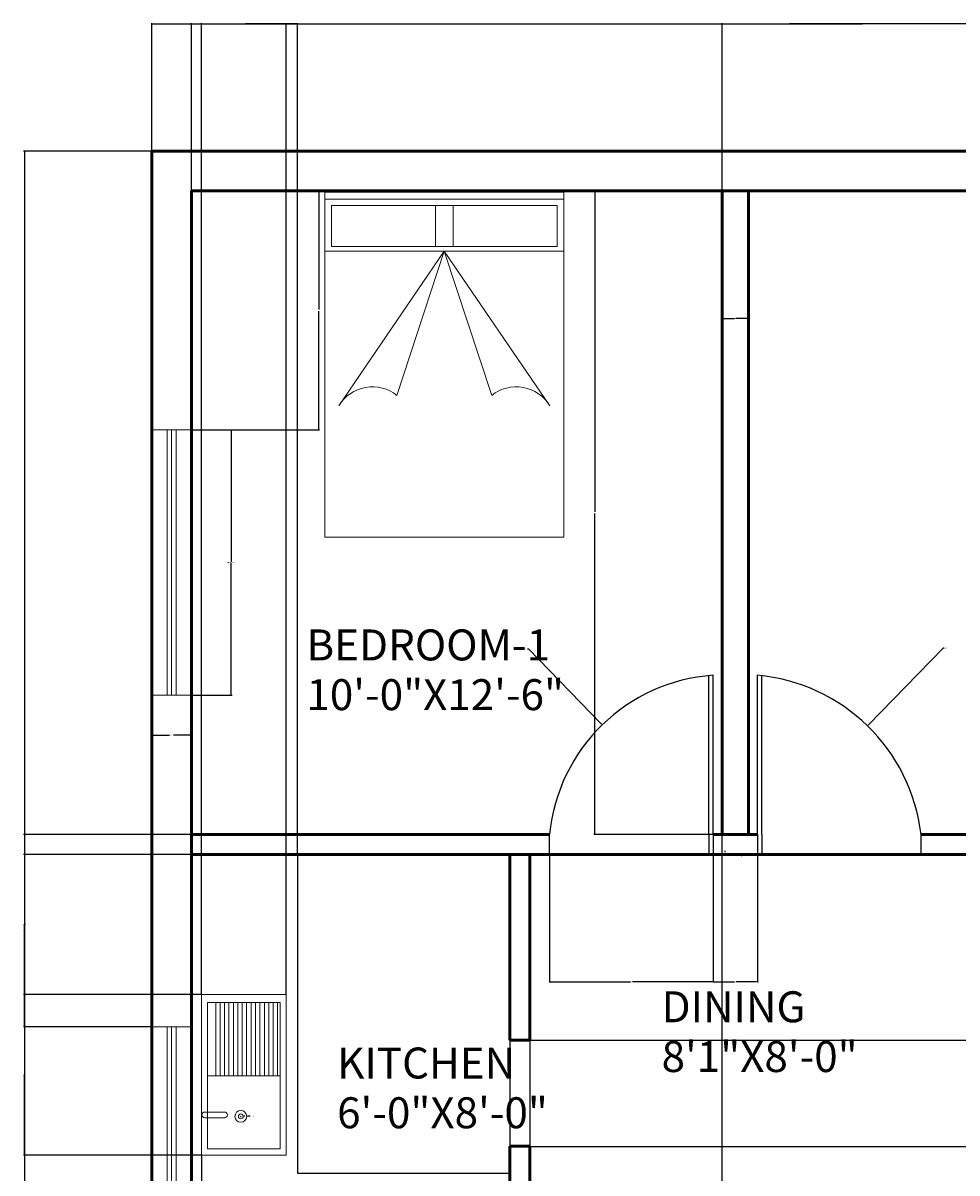
# Model space of a CAD drawing. Units: inches. Extents: x 2750 to 3097, y 1429 to 2028.
# Tile 3 of 4: x 2750 to 2962, y 1768 to 2028. Entities that reach past the tile are written whole.
import ezdxf

# ---------------------------------------------------------------- set-up
doc = ezdxf.new("R2010")
doc.units = ezdxf.units.IN
for name, color, linetype, lineweight in [('A-ANNO-DIMS', 2, 'Continuous', 18), ('A-AREA-IDEN', 7, 'Continuous', 25), ('A-DOOR', 3, 'Continuous', 25), ('A-FIXT-PATT', 252, 'Continuous', 13), ('A-FLOR-CASE', 8, 'Continuous', 25), ('A-FLOR-FIXT', 9, 'Continuous', 18), ('A-FURN', 8, 'Continuous', 18), ('A-GLAZ', 4, 'Continuous', 18), ('A-WALL', 7, 'Continuous', 50)]:
    doc.layers.add(name, color=color, linetype=linetype, lineweight=lineweight)
doc.styles.get("Standard").update_dxf_attribs({"font": 'arial.ttf'})
doc.dimstyles.get("Standard").update_dxf_attribs({"dimtxt": 0.18, "dimasz": 0.18, "dimexe": 0.18, "dimexo": 0.0625, "dimgap": 0.09, "dimtad": 0, "dimtih": 1, "dimtoh": 1, "dimdec": 4, "dimzin": 0, "dimdsep": 46, "dimtxsty": 'Standard', "dimcen": 0.09, "dimadec": 0, "dimazin": 0, "dimtfac": 1, "dimtdec": 4, "dimtofl": 0, "dimtmove": 0, "dimatfit": 3, "dimfxl": 1, "dimtolj": 1, "dimtzin": 0, "dimarcsym": 0})

# ---------------------------------------------------------------- blocks, each defined once
blk = doc.blocks.new('BED-DOUBLE-54X78')
for p, q in [((0, 78), (0, 0)), ((54, 78), (0, 78)), ((54, 0), (54, 78)), ((27, 13.39), (3.13, 48.31)), ((27, 13.39), (50.87, 48.31)), ((27, 13.39), (16.28, 45.98)), ((27, 13.39), (37.72, 45.98)), ((0, 13.39), (54, 13.39)), ((24.99, 3.04), (24.99, 12.35)), ((28.99, 3.04), (28.99, 12.35)), ((0, 1.59), (54, 1.59)), ((0, 0), (54, 0))]:
    blk.add_line(p, q)
blk.add_lwpolyline([(1.48, 3.04), (52.5, 3.04), (52.5, 12.35), (1.48, 12.35)], close=True)
for centre, start, end in [((10.73, 52.93), 211.2898, 308.6091), ((43.27, 52.93), 231.3909, 328.7102)]:
    blk.add_arc(centre, 8.89, start, end)
blk = doc.blocks.new('WIN-60IN')
for p, q in [((9, 60), (0, 60)), ((3.5, 60), (3.5, 0)), ((4.5, 60), (4.5, 0)), ((5.5, 60), (5.5, 0)), ((9, 0), (0, 0))]:
    blk.add_line(p, q)
blk = doc.blocks.new('WIN-36IN')
for p, q in [((9, 36), (0, 36)), ((3.5, 36), (3.5, 0)), ((4.5, 36), (4.5, 0)), ((5.5, 36), (5.5, 0)), ((9, 0), (0, 0))]:
    blk.add_line(p, q)
blk = doc.blocks.new('*D5')
at = {"layer": 'A-ANNO-DIMS', "color": 0, "lineweight": -2, "transparency": 16777216}
for p, q in [((2788.58, 1935.59), (2797.7, 1935.59)), ((2797.52, 1935.41), (2797.52, 1905.78)), ((2797.52, 1875.77), (2797.52, 1905.41)), ((2788.58, 1875.59), (2797.7, 1875.59))]:
    blk.add_line(p, q, dxfattribs=at)
at = {"layer": 'A-ANNO-DIMS', "color": 0, "transparency": 16777216}
for points in [[(2797.49, 1935.41), (2797.55, 1935.41), (2797.52, 1935.59)], [(2797.49, 1875.77), (2797.55, 1875.77), (2797.52, 1875.59)]]:
    blk.add_solid(points, dxfattribs=at)
at = {"layer": 'Defpoints', "color": 0, "transparency": 16777216}
for p in [(2788.52, 1935.59), (2797.52, 1935.59), (2788.52, 1875.59)]:
    blk.add_point(p, dxfattribs=at)
at = {"layer": 'A-ANNO-DIMS', "color": 0, "transparency": 16777216, "insert": (2797.52, 1905.59), "char_height": 0.18, "attachment_point": 5}
blk.add_mtext('\\A1;WINDOW 60 TYP.', dxfattribs=at)
blk = doc.blocks.new('*D6')
at = {"layer": 'A-ANNO-DIMS', "color": 0, "lineweight": -2, "transparency": 16777216}
for p, q in [((2779.52, 1875.53), (2779.52, 1866.41)), ((2788.52, 1875.53), (2788.52, 1866.41)), ((2779.7, 1866.59), (2783.56, 1866.59)), ((2788.34, 1866.59), (2784.48, 1866.59))]:
    blk.add_line(p, q, dxfattribs=at)
at = {"layer": 'A-ANNO-DIMS', "color": 0, "transparency": 16777216}
for points in [[(2779.7, 1866.62), (2779.7, 1866.56), (2779.52, 1866.59)], [(2788.34, 1866.62), (2788.34, 1866.56), (2788.52, 1866.59)]]:
    blk.add_solid(points, dxfattribs=at)
at = {"layer": 'Defpoints', "color": 0, "transparency": 16777216}
for p in [(2779.52, 1875.59), (2788.52, 1875.59), (2788.52, 1866.59)]:
    blk.add_point(p, dxfattribs=at)
at = {"layer": 'A-ANNO-DIMS', "color": 0, "transparency": 16777216, "insert": (2784.02, 1866.59), "char_height": 0.18, "attachment_point": 5}
blk.add_mtext('\\A1;9 TYP.', dxfattribs=at)
blk = doc.blocks.new('*D13')
at = {"layer": 'A-ANNO-DIMS', "color": 0, "lineweight": -2, "transparency": 16777216}
for p, q in [((2779.52, 1998.66), (2779.52, 2027.57)), ((2779.7, 2027.39), (2923.23, 2027.39)), ((3067.34, 2027.39), (2923.81, 2027.39)), ((3067.52, 1998.66), (3067.52, 2027.57))]:
    blk.add_line(p, q, dxfattribs=at)
at = {"layer": 'A-ANNO-DIMS', "color": 0, "transparency": 16777216}
for points in [[(2779.7, 2027.42), (2779.7, 2027.36), (2779.52, 2027.39)], [(3067.34, 2027.42), (3067.34, 2027.36), (3067.52, 2027.39)]]:
    blk.add_solid(points, dxfattribs=at)
at = {"layer": 'Defpoints', "color": 0, "transparency": 16777216}
for p in [(3067.52, 2027.39), (2779.52, 1998.59), (3067.52, 1998.59)]:
    blk.add_point(p, dxfattribs=at)
at = {"layer": 'A-ANNO-DIMS', "color": 0, "transparency": 16777216, "insert": (2923.52, 2027.39), "char_height": 0.18, "attachment_point": 5}
blk.add_mtext('\\A1;288', dxfattribs=at)
blk = doc.blocks.new('*D14')
at = {"layer": 'A-ANNO-DIMS', "color": 0, "lineweight": -2, "transparency": 16777216}
for p, q in [((2779.46, 1998.59), (2750.54, 1998.59)), ((2750.72, 1998.41), (2750.72, 1734.77)), ((2750.72, 1470.77), (2750.72, 1734.41)), ((2906.46, 1470.59), (2750.54, 1470.59))]:
    blk.add_line(p, q, dxfattribs=at)
at = {"layer": 'A-ANNO-DIMS', "color": 0, "transparency": 16777216}
for points in [[(2750.69, 1998.41), (2750.75, 1998.41), (2750.72, 1998.59)], [(2750.69, 1470.77), (2750.75, 1470.77), (2750.72, 1470.59)]]:
    blk.add_solid(points, dxfattribs=at)
at = {"layer": 'Defpoints', "color": 0, "transparency": 16777216}
for p in [(2750.72, 1998.59), (2779.52, 1998.59), (2906.52, 1470.59)]:
    blk.add_point(p, dxfattribs=at)
at = {"layer": 'A-ANNO-DIMS', "color": 0, "transparency": 16777216, "insert": (2750.72, 1734.59), "char_height": 0.18, "attachment_point": 5}
blk.add_mtext('\\A1;528', dxfattribs=at)
blk = doc.blocks.new('*D22')
at = {"layer": 'A-ANNO-DIMS', "color": 0, "lineweight": -2, "transparency": 16777216}
for p, q in [((2788.46, 1844.09), (2750.54, 1844.09)), ((2750.72, 1843.91), (2750.72, 1822.52)), ((2750.72, 1800.77), (2750.72, 1822.16)), ((2779.46, 1800.59), (2750.54, 1800.59))]:
    blk.add_line(p, q, dxfattribs=at)
at = {"layer": 'A-ANNO-DIMS', "color": 0, "transparency": 16777216}
for points in [[(2750.69, 1843.91), (2750.75, 1843.91), (2750.72, 1844.09)], [(2750.69, 1800.77), (2750.75, 1800.77), (2750.72, 1800.59)]]:
    blk.add_solid(points, dxfattribs=at)
at = {"layer": 'Defpoints', "color": 0, "transparency": 16777216}
for p in [(2788.52, 1844.09), (2750.72, 1800.59), (2779.52, 1800.59)]:
    blk.add_point(p, dxfattribs=at)
at = {"layer": 'A-ANNO-DIMS', "color": 0, "transparency": 16777216, "insert": (2750.72, 1822.34), "char_height": 0.18, "attachment_point": 5}
blk.add_mtext('\\A1;43.5', dxfattribs=at)
blk = doc.blocks.new('*D23')
at = {"layer": 'A-ANNO-DIMS', "color": 0, "lineweight": -2, "transparency": 16777216}
for p, q in [((2788.58, 1989.59), (2817.5, 1989.59)), ((2817.32, 1989.41), (2817.32, 1962.77)), ((2817.32, 1935.77), (2817.32, 1962.41)), ((2788.58, 1935.59), (2817.5, 1935.59))]:
    blk.add_line(p, q, dxfattribs=at)
at = {"layer": 'A-ANNO-DIMS', "color": 0, "transparency": 16777216}
for points in [[(2817.29, 1989.41), (2817.35, 1989.41), (2817.32, 1989.59)], [(2817.29, 1935.77), (2817.35, 1935.77), (2817.32, 1935.59)]]:
    blk.add_solid(points, dxfattribs=at)
at = {"layer": 'Defpoints', "color": 0, "transparency": 16777216}
for p in [(2788.52, 1989.59), (2788.52, 1935.59), (2817.32, 1935.59)]:
    blk.add_point(p, dxfattribs=at)
at = {"layer": 'A-ANNO-DIMS', "color": 0, "transparency": 16777216, "insert": (2817.32, 1962.59), "char_height": 0.18, "attachment_point": 5}
blk.add_mtext('\\A1;54', dxfattribs=at)
blk = doc.blocks.new('*D30')
at = {"layer": 'A-ANNO-DIMS', "color": 0, "lineweight": -2, "transparency": 16777216}
for p, q in [((2908.46, 1989.59), (2879.54, 1989.59)), ((2879.72, 1989.41), (2879.72, 1917.02)), ((2879.72, 1844.27), (2879.72, 1916.66)), ((2908.46, 1844.09), (2879.54, 1844.09))]:
    blk.add_line(p, q, dxfattribs=at)
at = {"layer": 'A-ANNO-DIMS', "color": 0, "transparency": 16777216}
for points in [[(2879.69, 1989.41), (2879.75, 1989.41), (2879.72, 1989.59)], [(2879.69, 1844.27), (2879.75, 1844.27), (2879.72, 1844.09)]]:
    blk.add_solid(points, dxfattribs=at)
at = {"layer": 'Defpoints', "color": 0, "transparency": 16777216}
for p in [(2879.72, 1989.59), (2908.52, 1989.59), (2908.52, 1844.09)]:
    blk.add_point(p, dxfattribs=at)
at = {"layer": 'A-ANNO-DIMS', "color": 0, "transparency": 16777216, "insert": (2879.72, 1916.84), "char_height": 0.18, "attachment_point": 5}
blk.add_mtext('\\A1;145.5', dxfattribs=at)
blk = doc.blocks.new('*D33')
at = {"layer": 'A-ANNO-DIMS', "color": 0, "lineweight": -2, "transparency": 16777216}
for p, q in [((2908.52, 1989.53), (2908.52, 1960.61)), ((2914.52, 1989.53), (2914.52, 1960.61)), ((2908.7, 1960.79), (2911.37, 1960.79)), ((2914.34, 1960.79), (2911.67, 1960.79))]:
    blk.add_line(p, q, dxfattribs=at)
at = {"layer": 'A-ANNO-DIMS', "color": 0, "transparency": 16777216}
for points in [[(2908.7, 1960.82), (2908.7, 1960.76), (2908.52, 1960.79)], [(2914.34, 1960.82), (2914.34, 1960.76), (2914.52, 1960.79)]]:
    blk.add_solid(points, dxfattribs=at)
at = {"layer": 'Defpoints', "color": 0, "transparency": 16777216}
for p in [(2908.52, 1989.59), (2914.52, 1989.59), (2908.52, 1960.79)]:
    blk.add_point(p, dxfattribs=at)
at = {"layer": 'A-ANNO-DIMS', "color": 0, "transparency": 16777216, "insert": (2911.52, 1960.79), "char_height": 0.18, "attachment_point": 5}
blk.add_mtext('\\A1;6', dxfattribs=at)
blk = doc.blocks.new('*D34')
at = {"layer": 'A-ANNO-DIMS', "color": 0, "lineweight": -2, "transparency": 16777216}
for p, q in [((2869.52, 1839.53), (2869.52, 1810.61)), ((2906.52, 1839.53), (2906.52, 1810.61)), ((2869.7, 1810.79), (2887.8, 1810.79)), ((2906.34, 1810.79), (2888.24, 1810.79))]:
    blk.add_line(p, q, dxfattribs=at)
at = {"layer": 'A-ANNO-DIMS', "color": 0, "transparency": 16777216}
for points in [[(2869.7, 1810.82), (2869.7, 1810.76), (2869.52, 1810.79)], [(2906.34, 1810.82), (2906.34, 1810.76), (2906.52, 1810.79)]]:
    blk.add_solid(points, dxfattribs=at)
at = {"layer": 'Defpoints', "color": 0, "transparency": 16777216}
for p in [(2869.52, 1839.59), (2906.52, 1839.59), (2869.52, 1810.79)]:
    blk.add_point(p, dxfattribs=at)
at = {"layer": 'A-ANNO-DIMS', "color": 0, "transparency": 16777216, "insert": (2888.02, 1810.79), "char_height": 0.18, "attachment_point": 5}
blk.add_mtext('\\A1;37', dxfattribs=at)
blk = doc.blocks.new('*D35')
at = {"layer": 'A-ANNO-DIMS', "color": 0, "lineweight": -2, "transparency": 16777216}
for p, q in [((2906.52, 1839.53), (2906.52, 1810.61)), ((2916.52, 1839.53), (2916.52, 1810.61)), ((2906.7, 1810.79), (2911.31, 1810.79)), ((2916.34, 1810.79), (2911.73, 1810.79))]:
    blk.add_line(p, q, dxfattribs=at)
at = {"layer": 'A-ANNO-DIMS', "color": 0, "transparency": 16777216}
for points in [[(2906.7, 1810.82), (2906.7, 1810.76), (2906.52, 1810.79)], [(2916.34, 1810.82), (2916.34, 1810.76), (2916.52, 1810.79)]]:
    blk.add_solid(points, dxfattribs=at)
at = {"layer": 'Defpoints', "color": 0, "transparency": 16777216}
for p in [(2906.52, 1839.59), (2916.52, 1839.59), (2906.52, 1810.79)]:
    blk.add_point(p, dxfattribs=at)
at = {"layer": 'A-ANNO-DIMS', "color": 0, "transparency": 16777216, "insert": (2911.52, 1810.79), "char_height": 0.18, "attachment_point": 5}
blk.add_mtext('\\A1;10', dxfattribs=at)
blk = doc.blocks.new('*D38')
at = {"layer": 'A-ANNO-DIMS', "color": 0, "lineweight": -2, "transparency": 16777216}
for p, q in [((2788.52, 1839.66), (2788.52, 2027.57)), ((2788.7, 2027.39), (2800.3, 2027.39)), ((2812.34, 2027.39), (2800.74, 2027.39)), ((2812.52, 1839.66), (2812.52, 2027.57))]:
    blk.add_line(p, q, dxfattribs=at)
at = {"layer": 'A-ANNO-DIMS', "color": 0, "transparency": 16777216}
for points in [[(2788.7, 2027.42), (2788.7, 2027.36), (2788.52, 2027.39)], [(2812.34, 2027.42), (2812.34, 2027.36), (2812.52, 2027.39)]]:
    blk.add_solid(points, dxfattribs=at)
at = {"layer": 'Defpoints', "color": 0, "transparency": 16777216}
for p in [(2812.52, 2027.39), (2788.52, 1839.59), (2812.52, 1839.59)]:
    blk.add_point(p, dxfattribs=at)
at = {"layer": 'A-ANNO-DIMS', "color": 0, "transparency": 16777216, "insert": (2800.52, 2027.39), "char_height": 0.18, "attachment_point": 5}
blk.add_mtext('\\A1;24', dxfattribs=at)
blk = doc.blocks.new('*D40')
at = {"layer": 'A-ANNO-DIMS', "color": 0, "lineweight": -2, "transparency": 16777216}
for p, q in [((2860.58, 1797.59), (3096.5, 1797.59)), ((3096.32, 1797.41), (3096.32, 1785.77)), ((3096.32, 1773.77), (3096.32, 1785.41)), ((2860.58, 1773.59), (3096.5, 1773.59))]:
    blk.add_line(p, q, dxfattribs=at)
at = {"layer": 'A-ANNO-DIMS', "color": 0, "transparency": 16777216}
for points in [[(3096.29, 1797.41), (3096.35, 1797.41), (3096.32, 1797.59)], [(3096.29, 1773.77), (3096.35, 1773.77), (3096.32, 1773.59)]]:
    blk.add_solid(points, dxfattribs=at)
at = {"layer": 'Defpoints', "color": 0, "transparency": 16777216}
for p in [(2860.52, 1797.59), (3096.32, 1797.59), (2860.52, 1773.59)]:
    blk.add_point(p, dxfattribs=at)
at = {"layer": 'A-ANNO-DIMS', "color": 0, "transparency": 16777216, "insert": (3096.32, 1785.59), "char_height": 0.18, "attachment_point": 5}
blk.add_mtext('\\A1;24', dxfattribs=at)
blk = doc.blocks.new('*D41')
at = {"layer": 'A-ANNO-DIMS', "color": 0, "lineweight": -2, "transparency": 16777216}
for p, q in [((2865.08, 1839.59), (3096.5, 1839.59)), ((3096.32, 1839.41), (3096.32, 1818.77)), ((3096.32, 1797.77), (3096.32, 1818.41)), ((2865.08, 1797.59), (3096.5, 1797.59))]:
    blk.add_line(p, q, dxfattribs=at)
at = {"layer": 'A-ANNO-DIMS', "color": 0, "transparency": 16777216}
for points in [[(3096.29, 1839.41), (3096.35, 1839.41), (3096.32, 1839.59)], [(3096.29, 1797.77), (3096.35, 1797.77), (3096.32, 1797.59)]]:
    blk.add_solid(points, dxfattribs=at)
at = {"layer": 'Defpoints', "color": 0, "transparency": 16777216}
for p in [(2865.02, 1839.59), (3096.32, 1839.59), (2865.02, 1797.59)]:
    blk.add_point(p, dxfattribs=at)
at = {"layer": 'A-ANNO-DIMS', "color": 0, "transparency": 16777216, "insert": (3096.32, 1818.59), "char_height": 0.18, "attachment_point": 5}
blk.add_mtext('\\A1;42', dxfattribs=at)
blk = doc.blocks.new('*D42')
at = {"layer": 'A-ANNO-DIMS', "color": 0, "lineweight": -2, "transparency": 16777216}
for p, q in [((2860.52, 1797.53), (2860.52, 1441.61)), ((2865.02, 1797.53), (2865.02, 1441.61)), ((2860.7, 1441.79), (2862.51, 1441.79)), ((2864.84, 1441.79), (2863.03, 1441.79))]:
    blk.add_line(p, q, dxfattribs=at)
at = {"layer": 'A-ANNO-DIMS', "color": 0, "transparency": 16777216}
for points in [[(2860.7, 1441.82), (2860.7, 1441.76), (2860.52, 1441.79)], [(2864.84, 1441.82), (2864.84, 1441.76), (2865.02, 1441.79)]]:
    blk.add_solid(points, dxfattribs=at)
at = {"layer": 'Defpoints', "color": 0, "transparency": 16777216}
for p in [(2860.52, 1797.59), (2865.02, 1797.59), (2865.02, 1441.79)]:
    blk.add_point(p, dxfattribs=at)
at = {"layer": 'A-ANNO-DIMS', "color": 0, "transparency": 16777216, "insert": (2862.77, 1441.79), "char_height": 0.18, "attachment_point": 5}
blk.add_mtext('\\A1;4.5', dxfattribs=at)
blk = doc.blocks.new('*D43')
at = {"layer": 'A-ANNO-DIMS', "color": 0, "lineweight": -2, "transparency": 16777216}
for p, q in [((2790.76, 1807.98), (2790.76, 2027.57)), ((2790.94, 2027.39), (2799.89, 2027.39)), ((2809.75, 2027.39), (2800.8, 2027.39)), ((2809.93, 1807.98), (2809.93, 2027.57))]:
    blk.add_line(p, q, dxfattribs=at)
at = {"layer": 'A-ANNO-DIMS', "color": 0, "transparency": 16777216}
for points in [[(2790.94, 2027.42), (2790.94, 2027.36), (2790.76, 2027.39)], [(2809.75, 2027.42), (2809.75, 2027.36), (2809.93, 2027.39)]]:
    blk.add_solid(points, dxfattribs=at)
at = {"layer": 'Defpoints', "color": 0, "transparency": 16777216}
for p in [(2809.93, 2027.39), (2790.76, 1807.91), (2809.93, 1807.91)]:
    blk.add_point(p, dxfattribs=at)
at = {"layer": 'A-ANNO-DIMS', "color": 0, "transparency": 16777216, "insert": (2800.34, 2027.39), "char_height": 0.18, "attachment_point": 5}
blk.add_mtext('\\A1;19.165', dxfattribs=at)
blk = doc.blocks.new('*D44')
at = {"layer": 'A-ANNO-DIMS', "color": 0, "lineweight": -2, "transparency": 16777216}
for p, q in [((2790.7, 1807.91), (2750.54, 1807.91)), ((2750.72, 1807.73), (2750.72, 1789.94)), ((2750.72, 1771.79), (2750.72, 1789.58)), ((2790.7, 1771.61), (2750.54, 1771.61))]:
    blk.add_line(p, q, dxfattribs=at)
at = {"layer": 'A-ANNO-DIMS', "color": 0, "transparency": 16777216}
for points in [[(2750.69, 1807.73), (2750.75, 1807.73), (2750.72, 1807.91)], [(2750.69, 1771.79), (2750.75, 1771.79), (2750.72, 1771.61)]]:
    blk.add_solid(points, dxfattribs=at)
at = {"layer": 'Defpoints', "color": 0, "transparency": 16777216}
for p in [(2750.72, 1807.91), (2790.76, 1807.91), (2790.76, 1771.61)]:
    blk.add_point(p, dxfattribs=at)
at = {"layer": 'A-ANNO-DIMS', "color": 0, "transparency": 16777216, "insert": (2750.72, 1789.76), "char_height": 0.18, "attachment_point": 5}
blk.add_mtext('\\A1;36.31', dxfattribs=at)
blk = doc.blocks.new('*D45')
at = {"layer": 'A-ANNO-DIMS', "color": 0, "lineweight": -2, "transparency": 16777216}
for p, q in [((2788.46, 1839.59), (2750.54, 1839.59)), ((2750.72, 1839.41), (2750.72, 1823.94)), ((2750.72, 1808.09), (2750.72, 1823.57)), ((2790.7, 1807.91), (2750.54, 1807.91))]:
    blk.add_line(p, q, dxfattribs=at)
at = {"layer": 'A-ANNO-DIMS', "color": 0, "transparency": 16777216}
for points in [[(2750.69, 1839.41), (2750.75, 1839.41), (2750.72, 1839.59)], [(2750.69, 1808.09), (2750.75, 1808.09), (2750.72, 1807.91)]]:
    blk.add_solid(points, dxfattribs=at)
at = {"layer": 'Defpoints', "color": 0, "transparency": 16777216}
for p in [(2788.52, 1839.59), (2750.72, 1807.91), (2790.76, 1807.91)]:
    blk.add_point(p, dxfattribs=at)
at = {"layer": 'A-ANNO-DIMS', "color": 0, "transparency": 16777216, "insert": (2750.72, 1823.75), "char_height": 0.18, "attachment_point": 5}
blk.add_mtext('\\A1;31.68', dxfattribs=at)
blk = doc.blocks.new('*D46')
at = {"layer": 'A-ANNO-DIMS', "color": 0, "lineweight": -2, "transparency": 16777216}
for p, q in [((2790.76, 1771.54), (2790.76, 1441.61)), ((2788.52, 1764.53), (2788.52, 1441.61)), ((2788.7, 1441.79), (2789.32, 1441.79)), ((2790.58, 1441.79), (2789.97, 1441.79))]:
    blk.add_line(p, q, dxfattribs=at)
at = {"layer": 'A-ANNO-DIMS', "color": 0, "transparency": 16777216}
for points in [[(2788.7, 1441.82), (2788.7, 1441.76), (2788.52, 1441.79)], [(2790.58, 1441.82), (2790.58, 1441.76), (2790.76, 1441.79)]]:
    blk.add_solid(points, dxfattribs=at)
at = {"layer": 'Defpoints', "color": 0, "transparency": 16777216}
for p in [(2790.76, 1771.61), (2788.52, 1764.59), (2790.76, 1441.79)]:
    blk.add_point(p, dxfattribs=at)
at = {"layer": 'A-ANNO-DIMS', "color": 0, "transparency": 16777216, "insert": (2789.64, 1441.79), "char_height": 0.18, "attachment_point": 5}
blk.add_mtext('\\A1;2.24', dxfattribs=at)
blk = doc.blocks.new('*D52')
at = {"layer": 'A-ANNO-DIMS', "color": 0, "lineweight": -2, "transparency": 16777216}
for p, q in [((2908.52, 1605.66), (2908.52, 2027.57)), ((2908.7, 2027.39), (2940.3, 2027.39)), ((2972.34, 2027.39), (2940.74, 2027.39)), ((2972.52, 1605.66), (2972.52, 2027.57))]:
    blk.add_line(p, q, dxfattribs=at)
at = {"layer": 'A-ANNO-DIMS', "color": 0, "transparency": 16777216}
for points in [[(2908.7, 2027.42), (2908.7, 2027.36), (2908.52, 2027.39)], [(2972.34, 2027.42), (2972.34, 2027.36), (2972.52, 2027.39)]]:
    blk.add_solid(points, dxfattribs=at)
at = {"layer": 'Defpoints', "color": 0, "transparency": 16777216}
for p in [(2972.52, 2027.39), (2908.52, 1605.59), (2972.52, 1605.59)]:
    blk.add_point(p, dxfattribs=at)
at = {"layer": 'A-ANNO-DIMS', "color": 0, "transparency": 16777216, "insert": (2940.52, 2027.39), "char_height": 0.18, "attachment_point": 5}
blk.add_mtext('\\A1;64', dxfattribs=at)
blk = doc.blocks.new('*D59')
at = {"layer": 'A-ANNO-DIMS', "color": 0, "lineweight": -2, "transparency": 16777216}
for p, q in [((2958.53, 1886.26), (2941.54, 1868.8)), ((2958.71, 1886.26), (2958.53, 1886.26)), ((2912.81, 1839.36), (2912.99, 1839.36)), ((2912.9, 1839.27), (2912.9, 1839.45))]:
    blk.add_line(p, q, dxfattribs=at)
at = {"layer": 'A-ANNO-DIMS', "color": 0, "transparency": 16777216}
blk.add_solid([(2941.52, 1868.82), (2941.57, 1868.78), (2941.42, 1868.67)], dxfattribs=at)
at = {"layer": 'Defpoints', "color": 0, "transparency": 16777216}
for p in [(2941.42, 1868.67), (2912.9, 1839.36)]:
    blk.add_point(p, dxfattribs=at)
at = {"layer": 'A-ANNO-DIMS', "color": 0, "transparency": 16777216, "insert": (2959.12, 1886.26), "char_height": 0.18, "attachment_point": 5}
blk.add_mtext('\\A1;R40.9', dxfattribs=at)
blk = doc.blocks.new('*D60')
at = {"layer": 'A-ANNO-DIMS', "color": 0, "lineweight": -2, "transparency": 16777216}
for p, q in [((2864.54, 1886.04), (2864.72, 1886.04)), ((2864.72, 1886.04), (2881.29, 1869.01)), ((2909.15, 1840.28), (2909.33, 1840.28)), ((2909.24, 1840.19), (2909.24, 1840.37))]:
    blk.add_line(p, q, dxfattribs=at)
at = {"layer": 'A-ANNO-DIMS', "color": 0, "transparency": 16777216}
blk.add_solid([(2881.31, 1869.03), (2881.27, 1868.99), (2881.41, 1868.88)], dxfattribs=at)
at = {"layer": 'Defpoints', "color": 0, "transparency": 16777216}
for p in [(2881.41, 1868.88), (2909.24, 1840.28)]:
    blk.add_point(p, dxfattribs=at)
at = {"layer": 'A-ANNO-DIMS', "color": 0, "transparency": 16777216, "insert": (2864.13, 1886.04), "char_height": 0.18, "attachment_point": 5}
blk.add_mtext('\\A1;R39.9', dxfattribs=at)
blk = doc.blocks.new('*D67')
at = {"layer": 'A-ANNO-DIMS', "color": 0, "lineweight": -2, "transparency": 16777216}
for p, q in [((2799.58, 1780.36), (2799.76, 1780.36)), ((2799.67, 1780.27), (2799.67, 1780.45)), ((2801.8, 1780.39), (2801.18, 1780.38))]:
    blk.add_line(p, q, dxfattribs=at)
at = {"layer": 'A-ANNO-DIMS', "color": 0, "transparency": 16777216}
blk.add_solid([(2801.18, 1780.41), (2801.18, 1780.35), (2801, 1780.38)], dxfattribs=at)
at = {"layer": 'Defpoints', "color": 0, "transparency": 16777216}
for p in [(2798.34, 1780.34), (2801, 1780.38)]:
    blk.add_point(p, dxfattribs=at)
at = {"layer": 'A-ANNO-DIMS', "color": 0, "transparency": 16777216, "insert": (2802.22, 1780.39), "char_height": 0.18, "attachment_point": 5}
blk.add_mtext('\\A1;∅2.66', dxfattribs=at)
blk = doc.blocks.new('*D68')
at = {"layer": 'A-ANNO-DIMS', "color": 0, "lineweight": -2, "transparency": 16777216}
for p, q in [((2799.58, 1780.36), (2799.76, 1780.36)), ((2799.67, 1780.27), (2799.67, 1780.45)), ((2800.58, 1780.39), (2800.4, 1780.39))]:
    blk.add_line(p, q, dxfattribs=at)
at = {"layer": 'A-ANNO-DIMS', "color": 0, "transparency": 16777216}
blk.add_solid([(2800.4, 1780.42), (2800.4, 1780.36), (2800.22, 1780.38)], dxfattribs=at)
at = {"layer": 'Defpoints', "color": 0, "transparency": 16777216}
for p in [(2799.12, 1780.34), (2800.22, 1780.38)]:
    blk.add_point(p, dxfattribs=at)
at = {"layer": 'A-ANNO-DIMS', "color": 0, "transparency": 16777216, "insert": (2801, 1780.39), "char_height": 0.18, "attachment_point": 5}
blk.add_mtext('\\A1;∅1.10', dxfattribs=at)

msp = doc.modelspace()

# ---------------------------------------------------------------- hatches: boundary and pattern name
at = {"layer": 'A-FIXT-PATT'}
h = msp.add_hatch(dxfattribs=at)
h.set_pattern_fill('ANSI31', color=256, scale=0.3149606, angle=45, style=0)
h.paths.add_polyline_path([(2793.1756, 1789.5616), (2808.1756, 1789.5616), (2808.1756, 1806.1191), (2793.1756, 1806.1191)])

# ---------------------------------------------------------------- linework, layer by layer
at = {"layer": 'A-DOOR'}
for p, q in [((2905.5201, 1844.0925), (2905.5201, 1880.0925)), ((2906.5201, 1844.0925), (2906.5201, 1880.0925)), ((2916.5201, 1844.0925), (2916.5201, 1880.0925)), ((2917.5201, 1844.0925), (2917.5201, 1880.0925)), ((2869.5201, 1839.5925), (2869.5201, 1844.0925)), ((2905.5201, 1844.0925), (2905.5201, 1839.5925)), ((2906.5201, 1844.0925), (2906.5201, 1839.5925)), ((2916.5201, 1844.0925), (2916.5201, 1839.5925)), ((2917.5201, 1844.0925), (2917.5201, 1839.5925)), ((2953.5201, 1839.5925), (2953.5201, 1844.0925)), ((2905.5201, 1839.5925), (2869.5201, 1839.5925)), ((2917.5201, 1839.5925), (2953.5201, 1839.5925))]:
    msp.add_line(p, q, dxfattribs=at)
for centre, radius, start, end in [((2909.2403, 1840.2829), 39.9025, 93.908995, 174.521356), ((2912.8987, 1839.3566), 40.8965, 6.649866, 84.919783)]:
    msp.add_arc(centre, radius, start, end, dxfattribs=at)
at = {"layer": 'A-FLOR-CASE'}
for p, q in [((2788.5201, 1839.5925), (2812.5201, 1839.5925)), ((2788.5201, 1839.5925), (2788.5201, 1815.5925)), ((2788.5201, 1839.5925), (2812.5201, 1839.5925)), ((2812.5201, 1839.5925), (2812.5201, 1767.5629)), ((2812.5201, 1767.5629), (2860.5201, 1767.5629))]:
    msp.add_line(p, q, dxfattribs=at)
at = {"layer": 'A-FLOR-FIXT'}
for p, q in [((2792.1775, 1789.5616), (2808.5798, 1789.5616)), ((2791.5203, 1781.3448), (2795.9949, 1781.3448)), ((2791.5203, 1781.3448), (2796.0603, 1781.3448)), ((2791.5203, 1780.0392), (2796.0603, 1780.0392)), ((2791.5203, 1780.0392), (2795.9949, 1780.0392))]:
    msp.add_line(p, q, dxfattribs=at)
for points in [[(2790.7618, 1807.9144), (2809.9266, 1807.9144), (2809.9266, 1771.6062), (2790.7618, 1771.6062)], [(2792.1775, 1806.1191), (2808.5798, 1806.1191), (2808.5798, 1773.0041), (2792.1775, 1773.0041)]]:
    msp.add_lwpolyline(points, close=True, dxfattribs=at)
for radius in [1.3318, 0.5481]:
    msp.add_circle((2799.6724, 1780.359), radius, dxfattribs=at)
for centre, start, end in [((2791.5203, 1780.692), 90, 270), ((2795.9949, 1780.692), 270, 90)]:
    msp.add_arc(centre, 0.6528, start, end, dxfattribs=at)
at = {"layer": 'A-GLAZ'}
for p, q in [((2784.0201, 1935.5925), (2788.5201, 1935.5925)), ((2784.0201, 1875.5925), (2788.5201, 1875.5925)), ((2784.0201, 1800.5925), (2788.5201, 1800.5925))]:
    msp.add_line(p, q, dxfattribs=at)
at = {"layer": 'A-WALL'}
for p, q in [((2779.5201, 1998.5925), (3067.5201, 1998.5925)), ((2779.5201, 1494.5925), (2779.5201, 1998.5925)), ((2788.5201, 1989.5925), (3058.5201, 1989.5925)), ((2788.5201, 1503.5925), (2788.5201, 1989.5925)), ((2908.5201, 1844.0925), (2908.5201, 1989.5925)), ((2914.5201, 1989.5925), (2914.5201, 1844.0925)), ((2788.5201, 1844.0925), (2869.5201, 1844.0925)), ((2908.5201, 1844.0925), (2906.5201, 1844.0925)), ((2906.5201, 1844.0925), (2916.5201, 1844.0925)), ((2914.5201, 1844.0925), (2916.5201, 1844.0925)), ((2953.5201, 1844.0925), (3058.5201, 1844.0925)), ((2788.5201, 1839.5925), (2965.0201, 1839.5925)), ((2860.5201, 1797.5925), (2860.5201, 1839.5925)), ((2865.0201, 1839.5925), (2865.0201, 1797.5925)), ((2865.0201, 1797.5925), (2865.0201, 1839.5925)), ((2865.0201, 1797.5925), (2860.5201, 1797.5925)), ((2860.5201, 1743.5925), (2860.5201, 1773.5925)), ((2860.5201, 1773.5925), (2865.0201, 1773.5925)), ((2865.0201, 1743.5925), (2865.0201, 1773.5925))]:
    msp.add_line(p, q, dxfattribs=at)

# ---------------------------------------------------------------- block references
at = {"layer": 'A-FURN', "rotation": 180}
msp.add_blockref('BED-DOUBLE-54X78', (2872.7026, 1989.3549), dxfattribs=at)
at = {"layer": 'A-GLAZ'}
for name, p in [('WIN-60IN', (2779.52, 1875.593)), ('WIN-36IN', (2779.52, 1764.593))]:
    msp.add_blockref(name, p, dxfattribs=at)

# ---------------------------------------------------------------- texts
at = {"layer": 'A-AREA-IDEN'}
for s, p in [('BEDROOM-1', (2814.5156, 1883.4577)), ('10\'-0"X12\'-6"', (2814.5156, 1872.2128)), ('DINING', (2894.848, 1801.639)), ('8\'1"X8\'-0"', (2894.848, 1790.3941)), ('KITCHEN', (2821.4628, 1788.9263)), ('6\'-0"X8\'-0"', (2821.4628, 1777.6814))]:
    msp.add_text(s, height=7, dxfattribs=at).set_placement(p)

# ---------------------------------------------------------------- dimensions: what is measured, and where the dimension line sits
at = {"layer": 'A-ANNO-DIMS'}
for base, p1, p2, override, picture, middle in [((3067.5201, 2027.3925), (2779.5201, 1998.5925), (3067.5201, 1998.5925), {"dimdec": 0, "dimlfac": 1, "dimrnd": 0, "dimzin": 0, "dimdsep": 46, "dimlunit": 2}, '*D13', (2923.5201, 2027.3925)), ((2812.5201, 2027.3925), (2788.5201, 1839.5925), (2812.5201, 1839.5925), {"dimdec": 0, "dimlfac": 1, "dimrnd": 0, "dimzin": 0, "dimdsep": 46, "dimlunit": 2}, '*D38', (2800.5201, 2027.3925)), ((2809.9266, 2027.3925), (2790.7618, 1807.9144), (2809.9266, 1807.9144), {"dimdec": 3, "dimlfac": 1, "dimrnd": 0, "dimzin": 0, "dimdsep": 46, "dimlunit": 2}, '*D43', (2800.3442, 2027.3925)), ((2972.5201, 2027.3925), (2908.5201, 1605.5925), (2972.5201, 1605.5925), {"dimdec": 0, "dimlfac": 1, "dimrnd": 0, "dimzin": 0, "dimdsep": 46, "dimlunit": 2}, '*D52', (2940.5201, 2027.3925)), ((2865.0201, 1441.7925), (2860.5201, 1797.5925), (2865.0201, 1797.5925), {"dimdec": 1, "dimlfac": 1, "dimrnd": 0, "dimzin": 0, "dimdsep": 46, "dimlunit": 2}, '*D42', (2862.7701, 1441.7925)), ((2790.7618, 1441.7925), (2788.5201, 1764.5925), (2790.7618, 1771.6062), {"dimdec": 2, "dimlfac": 1, "dimrnd": 0, "dimzin": 0, "dimdsep": 46, "dimlunit": 2}, '*D46', (2789.641, 1441.7925))]:
    dim = msp.add_linear_dim(base=base, p1=p1, p2=p2, dimstyle='Standard', override=override, dxfattribs=at)
    dim.commit()
    dim.dimension.update_dxf_attribs({"geometry": picture, "text_midpoint": middle})
for base, p1, p2, angle, override, picture, middle in [((2750.7201, 1998.5925), (2906.5201, 1470.5925), (2779.5201, 1998.5925), 90, {"dimdec": 0, "dimlfac": 1, "dimrnd": 0, "dimzin": 0, "dimdsep": 46, "dimlunit": 2}, '*D14', (2750.7201, 1734.5925)), ((2817.3201, 1935.5925), (2788.5201, 1989.5925), (2788.5201, 1935.5925), 270, {"dimdec": 0, "dimlfac": 1, "dimrnd": 0, "dimzin": 0, "dimdsep": 46, "dimlunit": 2}, '*D23', (2817.3201, 1962.5925)), ((2879.7201, 1989.5925), (2908.5201, 1844.0925), (2908.5201, 1989.5925), 90, {"dimdec": 1, "dimlfac": 1, "dimrnd": 0, "dimzin": 0, "dimdsep": 46, "dimlunit": 2}, '*D30', (2879.7201, 1916.8425)), ((2908.5201, 1960.7925), (2914.5201, 1989.5925), (2908.5201, 1989.5925), 180, {"dimdec": 0, "dimlfac": 1, "dimrnd": 0, "dimzin": 0, "dimdsep": 46, "dimlunit": 2}, '*D33', (2911.5201, 1960.7925)), ((2750.7201, 1800.5925), (2788.5201, 1844.0925), (2779.5201, 1800.5925), 90, {"dimdec": 1, "dimlfac": 1, "dimrnd": 0, "dimzin": 0, "dimdsep": 46, "dimlunit": 2}, '*D22', (2750.7201, 1822.3425)), ((2750.7201, 1807.9144), (2788.5201, 1839.5925), (2790.7618, 1807.9144), 90, {"dimdec": 2, "dimlfac": 1, "dimrnd": 0, "dimzin": 0, "dimdsep": 46, "dimlunit": 2}, '*D45', (2750.7201, 1823.7535)), ((3096.3201, 1839.5925), (2865.0201, 1797.5925), (2865.0201, 1839.5925), 90, {"dimdec": 0, "dimlfac": 1, "dimrnd": 0, "dimzin": 0, "dimdsep": 46, "dimlunit": 2}, '*D41', (3096.3201, 1818.5925)), ((2869.5201, 1810.7925), (2906.5201, 1839.5925), (2869.5201, 1839.5925), 180, {"dimdec": 0, "dimlfac": 1, "dimrnd": 0, "dimzin": 0, "dimdsep": 46, "dimlunit": 2}, '*D34', (2888.0201, 1810.7925)), ((2906.5201, 1810.7925), (2916.5201, 1839.5925), (2906.5201, 1839.5925), 180, {"dimdec": 0, "dimlfac": 1, "dimrnd": 0, "dimzin": 0, "dimdsep": 46, "dimlunit": 2}, '*D35', (2911.5201, 1810.7925)), ((2750.7201, 1807.9144), (2790.7618, 1771.6062), (2790.7618, 1807.9144), 90, {"dimdec": 2, "dimlfac": 1, "dimrnd": 0, "dimzin": 0, "dimdsep": 46, "dimlunit": 2}, '*D44', (2750.7201, 1789.7603)), ((3096.3201, 1797.5925), (2860.5201, 1773.5925), (2860.5201, 1797.5925), 90, {"dimdec": 0, "dimlfac": 1, "dimrnd": 0, "dimzin": 0, "dimdsep": 46, "dimlunit": 2}, '*D40', (3096.3201, 1785.5925))]:
    dim = msp.add_linear_dim(base=base, p1=p1, p2=p2, angle=angle, dimstyle='Standard', override=override, dxfattribs=at)
    dim.commit()
    dim.dimension.update_dxf_attribs({"geometry": picture, "text_midpoint": middle})
dim = msp.add_linear_dim(base=(2797.5201, 1935.5925), p1=(2788.5201, 1875.5925), p2=(2788.5201, 1935.5925), angle=90, text='WINDOW <> TYP.', dimstyle='Standard', override={"dimdec": 0, "dimlfac": 1, "dimrnd": 0, "dimzin": 0, "dimdsep": 46, "dimlunit": 2}, dxfattribs=at)
dim.commit()
dim.dimension.update_dxf_attribs({"geometry": '*D5', "text_midpoint": (2797.5201, 1905.5925)})
for center, mpoint, picture, middle in [((2909.2403, 1840.2829), (2881.414, 1868.8819), '*D60', (2864.1282, 1886.0414)), ((2912.8987, 1839.3566), (2941.4182, 1868.6682), '*D59', (2959.12, 1886.2551))]:
    dim = msp.add_radius_dim(center=center, mpoint=mpoint, dimstyle='Standard', override={"dimdec": 1, "dimlfac": 1, "dimrnd": 0, "dimzin": 0, "dimdsep": 46, "dimlunit": 2}, dxfattribs=at)
    dim.commit()
    dim.dimension.update_dxf_attribs({"geometry": picture, "text_midpoint": middle, "dimtype": 164})
dim = msp.add_linear_dim(base=(2788.5201, 1866.5925), p1=(2779.5201, 1875.5925), p2=(2788.5201, 1875.5925), text='<> TYP.', dimstyle='Standard', override={"dimdec": 0, "dimlfac": 1, "dimrnd": 0, "dimzin": 0, "dimdsep": 46, "dimlunit": 2}, dxfattribs=at)
dim.commit()
dim.dimension.update_dxf_attribs({"geometry": '*D6', "text_midpoint": (2784.0201, 1866.5925)})
for p1, p2, picture, middle in [((2798.3408, 1780.3386), (2801.004, 1780.3793), '*D67', (2801.803, 1780.3915)), ((2799.1247, 1780.3388), (2800.2201, 1780.3791), '*D68', (2800.5799, 1780.3923))]:
    dim = msp.add_diameter_dim_2p(p1=p1, p2=p2, dimstyle='Standard', override={"dimdec": 2, "dimlfac": 1, "dimrnd": 0, "dimzin": 0, "dimdsep": 46, "dimlunit": 2}, dxfattribs=at)
    dim.commit()
    dim.dimension.update_dxf_attribs({"geometry": picture, "text_midpoint": middle, "dimtype": 163})

doc.saveas('drawing.dxf')
